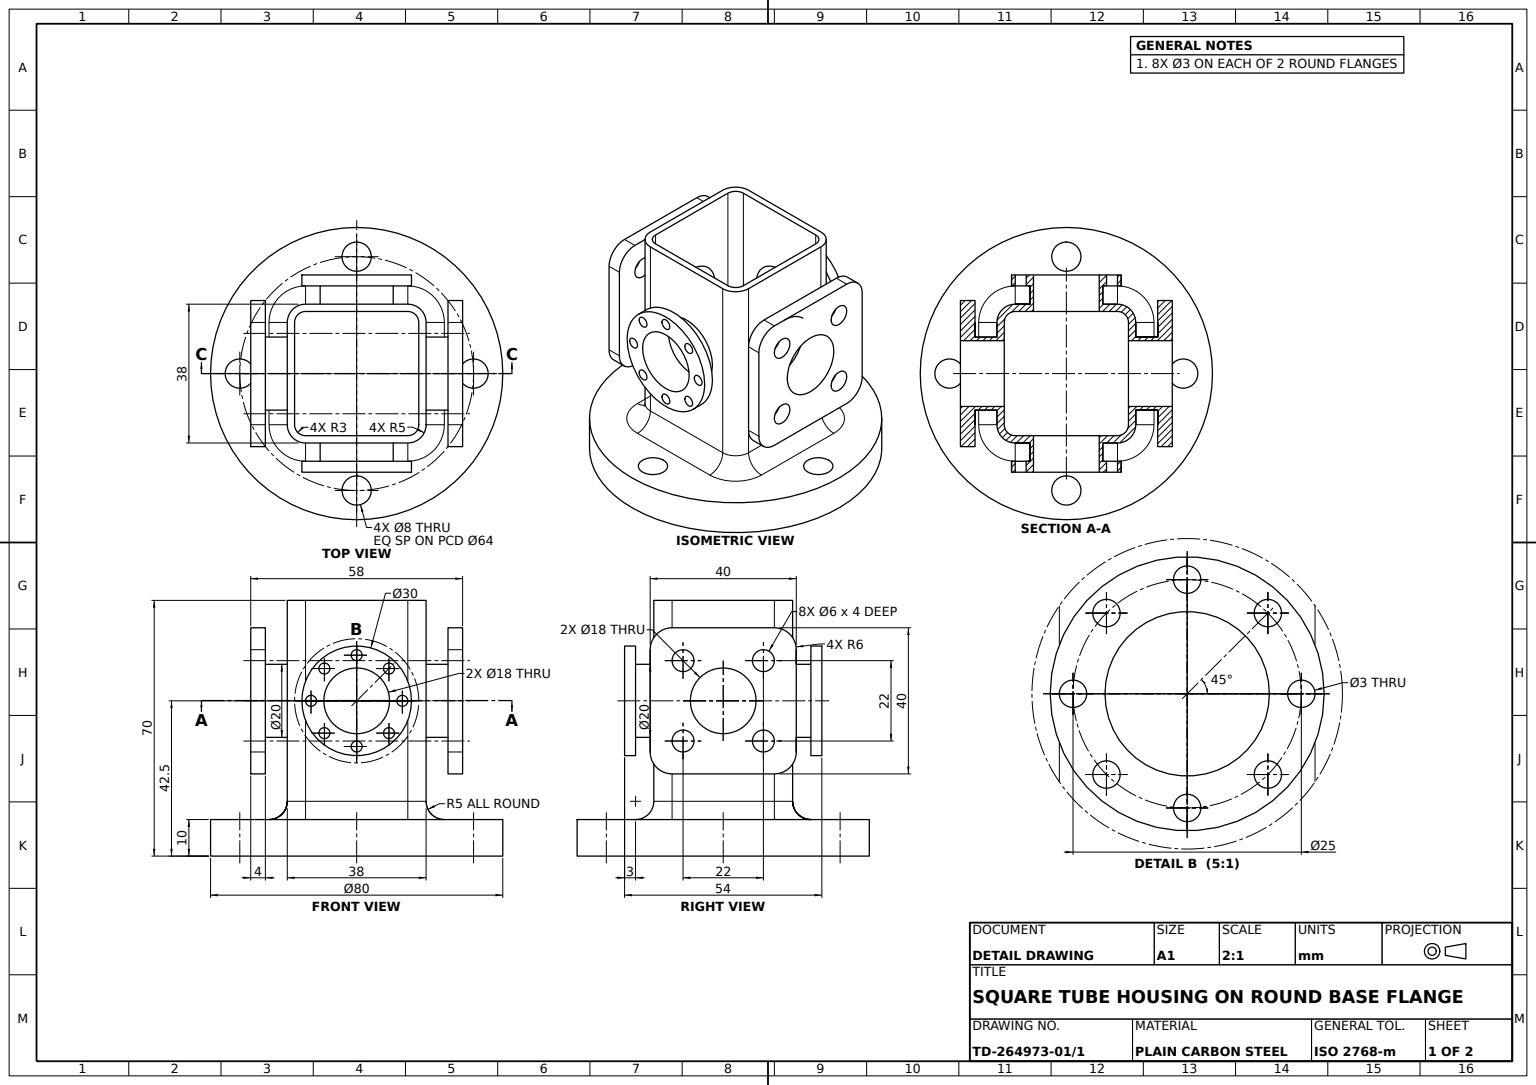
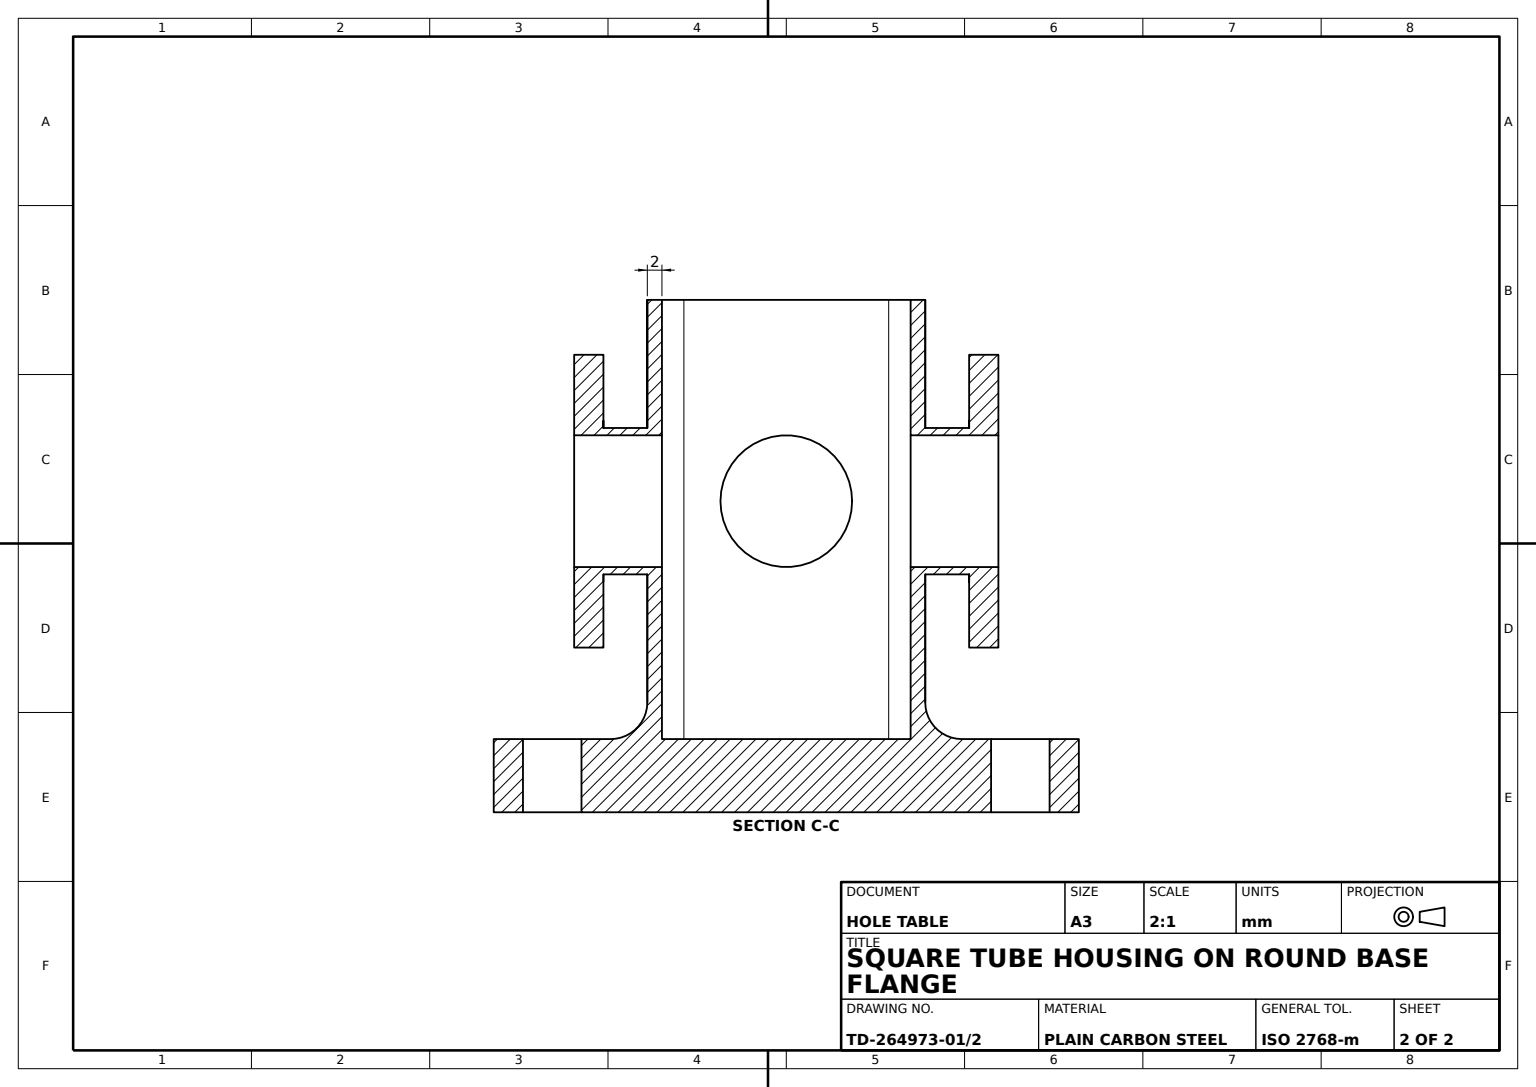
from build123d import *
from build123d.topology import SkipClean

# Parameters (mm, degrees)
BASE_FLANGE_SKETCH_R           = 40
BASE_FLANGE_SKETCH_R_2         = 4
BASE_FLANGE_80_DEPTH           = 10
SQUARE_BODY_38X38_WALL_2_DEPTH = 60
BODY_TO_FLANGE_FILLET_R5_R     = 5
CROSS_BORE_A_SKETCH_R          = 9
CROSS_BORE_A_18_DEPTH          = 60
CROSS_BORE_B_SKETCH_R          = 9
CROSS_BORE_B_18_DEPTH          = 60
PORT_START                     = 5
PORT_A1_STUB_SKETCH_R          = 10
PORT_A1_STUB_SKETCH_R_2        = 9
PORT_A1_STUB_18_DEPTH          = 5
ROUND_START                    = 3
ROUND_FLANGE_A1_SKETCH_R       = 15
ROUND_FLANGE_A1_SKETCH_R_2     = 9
ROUND_FLANGE_A1_SKETCH_R_3     = 1.5
ROUND_FLANGE_A1_30_DEPTH       = 3
PORT_A2_STUB_SKETCH_R          = 10
PORT_A2_STUB_SKETCH_R_2        = 9
PORT_A2_STUB_18_DEPTH          = 5
ROUND_FLANGE_A2_SKETCH_R       = 15
ROUND_FLANGE_A2_SKETCH_R_2     = 9
ROUND_FLANGE_A2_SKETCH_R_3     = 1.5
ROUND_FLANGE_A2_30_DEPTH       = 3
PORT_START_2                   = 6
PORT_B1_STUB_SKETCH_R          = 10
PORT_B1_STUB_SKETCH_R_2        = 9
PORT_B1_STUB_18_DEPTH          = 6
SQUARE_START                   = 4
SQUARE_FLANGE_B1_SKETCH_R      = 9
SQUARE_FLANGE_B1_SKETCH_R_2    = 3
SQUARE_FLANGE_B1_40X40_DEPTH   = 4
PORT_B2_STUB_SKETCH_R          = 10
PORT_B2_STUB_SKETCH_R_2        = 9
PORT_B2_STUB_18_DEPTH          = 6
SQUARE_FLANGE_B2_SKETCH_R      = 9
SQUARE_FLANGE_B2_SKETCH_R_2    = 3
SQUARE_FLANGE_B2_40X40_DEPTH   = 4


with BuildPart() as part:
    # Base Flange Sketch → Base Flange Ø80 (new body)
    with BuildSketch(Plane(origin=(0, 0, 0), x_dir=(1, 0, 0), z_dir=(0, 1, 0))):
        with Locations(Location((0, 0, 0), (0, 0, 270))):
            Circle(BASE_FLANGE_SKETCH_R)
        with Locations(Location((0, 32, 0), (0, 0, 270))):
            Circle(BASE_FLANGE_SKETCH_R_2, mode=Mode.SUBTRACT)
        with Locations(Location((32, 0, 0), (0, 0, 270))):
            Circle(BASE_FLANGE_SKETCH_R_2, mode=Mode.SUBTRACT)
        with Locations(Location((0, -32, 0), (0, 0, 270))):
            Circle(BASE_FLANGE_SKETCH_R_2, mode=Mode.SUBTRACT)
        with Locations(Location((-32, 0, 0), (0, 0, 270))):
            Circle(BASE_FLANGE_SKETCH_R_2, mode=Mode.SUBTRACT)
    extrude(amount=BASE_FLANGE_80_DEPTH)

    # Square Body Sketch → Square Body 38x38 Wall 2 (add)
    with BuildSketch(Plane(origin=(0, 10, 0), x_dir=(1, 0, 0), z_dir=(0, 1, 0))):
        with BuildLine():
            Line((19, 14), (19, -14))
            ThreePointArc((19, -14), (17.535533906, -17.535533906), (14, -19))
            Line((14, -19), (-14, -19))
            ThreePointArc((-14, -19), (-17.535533906, -17.535533906), (-19, -14))
            Line((-19, -14), (-19, 14))
            ThreePointArc((-19, 14), (-17.535533906, 17.535533906), (-14, 19))
            Line((-14, 19), (14, 19))
            ThreePointArc((14, 19), (17.535533906, 17.535533906), (19, 14))
        make_face()
        with BuildLine():
            Line((17, 14), (17, -14))
            ThreePointArc((17, -14), (16.121320344, -16.121320344), (14, -17))
            Line((14, -17), (-14, -17))
            ThreePointArc((-14, -17), (-16.121320344, -16.121320344), (-17, -14))
            Line((-17, -14), (-17, 14))
            ThreePointArc((-17, 14), (-16.121320344, 16.121320344), (-14, 17))
            Line((-14, 17), (14, 17))
            ThreePointArc((14, 17), (16.121320344, 16.121320344), (17, 14))
        make_face(mode=Mode.SUBTRACT)
    extrude(amount=SQUARE_BODY_38X38_WALL_2_DEPTH)

    # Body to Flange Fillet R5
    body_to_flange_fillet_r5_edges = [part.edges().sort_by_distance(p)[0] for p in [
        (17.535533906, 10, 17.535533906),
        (19, 10, 0),
        (17.535533906, 10, -17.535533906),
        (0, 10, -19),
        (-17.535533906, 10, -17.535533906),
        (-19, 10, 0),
        (-17.535533906, 10, 17.535533906),
        (0, 10, 19),
    ]]
    fillet(body_to_flange_fillet_r5_edges, radius=BODY_TO_FLANGE_FILLET_R5_R)

    # Cross Bore A Sketch → Cross Bore A Ø18 (cut)
    with BuildSketch(Plane.XY.offset(19)):
        with Locations((0, 42.5)):
            Circle(CROSS_BORE_A_SKETCH_R)
    extrude(amount=-CROSS_BORE_A_18_DEPTH, mode=Mode.SUBTRACT)

    # Cross Bore B Sketch → Cross Bore B Ø18 (cut)
    with BuildSketch(Plane.ZY.offset(19)):
        with Locations((0, 42.5)):
            Circle(CROSS_BORE_B_SKETCH_R)
    extrude(amount=-CROSS_BORE_B_18_DEPTH, mode=Mode.SUBTRACT)

    # Port A1 Stub Sketch → Port A1 Stub Ø18 (add)
    with BuildSketch(Plane.XY.offset(19).offset(PORT_START)):
        with Locations((0, 42.5)):
            Circle(PORT_A1_STUB_SKETCH_R)
        with Locations((0, 42.5)):
            Circle(PORT_A1_STUB_SKETCH_R_2, mode=Mode.SUBTRACT)
    extrude(amount=-PORT_A1_STUB_18_DEPTH)

    # Round Flange A1 Sketch → Round Flange A1 Ø30 (add)
    with BuildSketch(Plane.XY.offset(24).offset(ROUND_START)):
        with Locations((0, 42.5)):
            Circle(ROUND_FLANGE_A1_SKETCH_R)
        with Locations((0, 42.5)):
            Circle(ROUND_FLANGE_A1_SKETCH_R_2, mode=Mode.SUBTRACT)
        with Locations((0, 55)):
            Circle(ROUND_FLANGE_A1_SKETCH_R_3, mode=Mode.SUBTRACT)
        with Locations((8.838834765, 51.338834765)):
            Circle(ROUND_FLANGE_A1_SKETCH_R_3, mode=Mode.SUBTRACT)
        with Locations((12.5, 42.5)):
            Circle(ROUND_FLANGE_A1_SKETCH_R_3, mode=Mode.SUBTRACT)
        with Locations((8.838834765, 33.661165235)):
            Circle(ROUND_FLANGE_A1_SKETCH_R_3, mode=Mode.SUBTRACT)
        with Locations((0, 30)):
            Circle(ROUND_FLANGE_A1_SKETCH_R_3, mode=Mode.SUBTRACT)
        with Locations((-8.838834765, 33.661165235)):
            Circle(ROUND_FLANGE_A1_SKETCH_R_3, mode=Mode.SUBTRACT)
        with Locations((-12.5, 42.5)):
            Circle(ROUND_FLANGE_A1_SKETCH_R_3, mode=Mode.SUBTRACT)
        with Locations((-8.838834765, 51.338834765)):
            Circle(ROUND_FLANGE_A1_SKETCH_R_3, mode=Mode.SUBTRACT)
    extrude(amount=-ROUND_FLANGE_A1_30_DEPTH)

    # Port A2 Stub Sketch → Port A2 Stub Ø18 (add)
    with SkipClean():  # the faces are left unmerged after this step: merging them gives an invalid solid
        with BuildSketch(Plane(origin=(0, 0, -19), x_dir=(-1, 0, 0), z_dir=(0, 0, -1))):
            with Locations((0, 42.5)):
                Circle(PORT_A2_STUB_SKETCH_R)
            with Locations((0, 42.5)):
                Circle(PORT_A2_STUB_SKETCH_R_2, mode=Mode.SUBTRACT)
        extrude(amount=PORT_A2_STUB_18_DEPTH)

    # Round Flange A2 Sketch → Round Flange A2 Ø30 (add)
    with SkipClean():  # the faces are left unmerged after this step: merging them gives an invalid solid
        with BuildSketch(Plane(origin=(0, 0, -24), x_dir=(-1, 0, 0), z_dir=(0, 0, -1))):
            with Locations(Location((0, 42.5, 0), (0, 0, 180))):
                Circle(ROUND_FLANGE_A2_SKETCH_R)
            with Locations(Location((0, 42.5, 0), (0, 0, 180))):
                Circle(ROUND_FLANGE_A2_SKETCH_R_2, mode=Mode.SUBTRACT)
            with Locations(Location((0, 55, 0), (0, 0, 180))):
                Circle(ROUND_FLANGE_A2_SKETCH_R_3, mode=Mode.SUBTRACT)
            with Locations(Location((8.838834765, 51.338834765, 0), (0, 0, 180))):
                Circle(ROUND_FLANGE_A2_SKETCH_R_3, mode=Mode.SUBTRACT)
            with Locations(Location((12.5, 42.5, 0), (0, 0, 180))):
                Circle(ROUND_FLANGE_A2_SKETCH_R_3, mode=Mode.SUBTRACT)
            with Locations(Location((8.838834765, 33.661165235, 0), (0, 0, 180))):
                Circle(ROUND_FLANGE_A2_SKETCH_R_3, mode=Mode.SUBTRACT)
            with Locations(Location((0, 30, 0), (0, 0, 180))):
                Circle(ROUND_FLANGE_A2_SKETCH_R_3, mode=Mode.SUBTRACT)
            with Locations(Location((-8.838834765, 33.661165235, 0), (0, 0, 180))):
                Circle(ROUND_FLANGE_A2_SKETCH_R_3, mode=Mode.SUBTRACT)
            with Locations(Location((-12.5, 42.5, 0), (0, 0, 180))):
                Circle(ROUND_FLANGE_A2_SKETCH_R_3, mode=Mode.SUBTRACT)
            with Locations(Location((-8.838834765, 51.338834765, 0), (0, 0, 180))):
                Circle(ROUND_FLANGE_A2_SKETCH_R_3, mode=Mode.SUBTRACT)
        extrude(amount=ROUND_FLANGE_A2_30_DEPTH)

    # Port B1 Stub Sketch → Port B1 Stub Ø18 (add)
    with SkipClean():  # the faces are left unmerged after this step: merging them gives an invalid solid
        with BuildSketch(Plane.ZY.offset(19).offset(PORT_START_2)):
            with Locations((0, 42.5)):
                Circle(PORT_B1_STUB_SKETCH_R)
            with Locations((0, 42.5)):
                Circle(PORT_B1_STUB_SKETCH_R_2, mode=Mode.SUBTRACT)
        extrude(amount=-PORT_B1_STUB_18_DEPTH)

    # Square Flange B1 Sketch → Square Flange B1 40x40 (add)
    with SkipClean():  # the faces are left unmerged after this step: merging them gives an invalid solid
        with BuildSketch(Plane.ZY.offset(25).offset(SQUARE_START)):
            with BuildLine():
                Line((-14, 62.5), (14, 62.5))
                ThreePointArc((14, 62.5), (18.242640687, 60.742640687), (20, 56.5))
                Line((20, 56.5), (20, 28.5))
                ThreePointArc((20, 28.5), (18.242640687, 24.257359313), (14, 22.5))
                Line((14, 22.5), (-14, 22.5))
                ThreePointArc((-14, 22.5), (-18.242640687, 24.257359313), (-20, 28.5))
                Line((-20, 28.5), (-20, 56.5))
                ThreePointArc((-20, 56.5), (-18.242640687, 60.742640687), (-14, 62.5))
            make_face()
            with Locations((0, 42.5)):
                Circle(SQUARE_FLANGE_B1_SKETCH_R, mode=Mode.SUBTRACT)
            with Locations((-11, 53.5)):
                Circle(SQUARE_FLANGE_B1_SKETCH_R_2, mode=Mode.SUBTRACT)
            with Locations((11, 53.5)):
                Circle(SQUARE_FLANGE_B1_SKETCH_R_2, mode=Mode.SUBTRACT)
            with Locations((-11, 31.5)):
                Circle(SQUARE_FLANGE_B1_SKETCH_R_2, mode=Mode.SUBTRACT)
            with Locations((11, 31.5)):
                Circle(SQUARE_FLANGE_B1_SKETCH_R_2, mode=Mode.SUBTRACT)
        extrude(amount=-SQUARE_FLANGE_B1_40X40_DEPTH)

    # Port B2 Stub Sketch → Port B2 Stub Ø18 (add)
    with SkipClean():  # the faces are left unmerged after this step: merging them gives an invalid solid
        with BuildSketch(Plane(origin=(19, 0, 0), x_dir=(0, 0, -1), z_dir=(1, 0, 0))):
            with Locations((0, 42.5)):
                Circle(PORT_B2_STUB_SKETCH_R)
            with Locations((0, 42.5)):
                Circle(PORT_B2_STUB_SKETCH_R_2, mode=Mode.SUBTRACT)
        extrude(amount=PORT_B2_STUB_18_DEPTH)

    # Square Flange B2 Sketch → Square Flange B2 40x40 (add)
    with SkipClean():  # the faces are left unmerged after this step: merging them gives an invalid solid
        with BuildSketch(Plane(origin=(25, 0, 0), x_dir=(0, 0, -1), z_dir=(1, 0, 0))):
            with BuildLine():
                Line((-14, 62.5), (14, 62.5))
                ThreePointArc((14, 62.5), (18.242640687, 60.742640687), (20, 56.5))
                Line((20, 56.5), (20, 28.5))
                ThreePointArc((20, 28.5), (18.242640687, 24.257359313), (14, 22.5))
                Line((14, 22.5), (-14, 22.5))
                ThreePointArc((-14, 22.5), (-18.242640687, 24.257359313), (-20, 28.5))
                Line((-20, 28.5), (-20, 56.5))
                ThreePointArc((-20, 56.5), (-18.242640687, 60.742640687), (-14, 62.5))
            make_face()
            with Locations(Location((0, 42.5, 0), (0, 0, 180))):
                Circle(SQUARE_FLANGE_B2_SKETCH_R, mode=Mode.SUBTRACT)
            with Locations(Location((-11, 53.5, 0), (0, 0, 180))):
                Circle(SQUARE_FLANGE_B2_SKETCH_R_2, mode=Mode.SUBTRACT)
            with Locations(Location((-11, 31.5, 0), (0, 0, 180))):
                Circle(SQUARE_FLANGE_B2_SKETCH_R_2, mode=Mode.SUBTRACT)
            with Locations(Location((11, 31.5, 0), (0, 0, 180))):
                Circle(SQUARE_FLANGE_B2_SKETCH_R_2, mode=Mode.SUBTRACT)
            with Locations(Location((11, 53.5, 0), (0, 0, 180))):
                Circle(SQUARE_FLANGE_B2_SKETCH_R_2, mode=Mode.SUBTRACT)
        extrude(amount=SQUARE_FLANGE_B2_40X40_DEPTH)


solid = part.part
